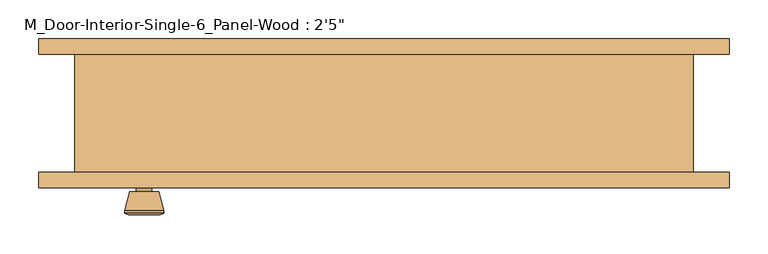
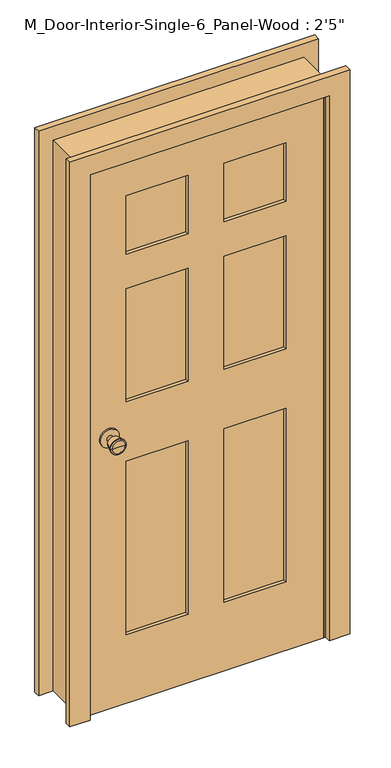
"""IFC4 building model written with IfcOpenShell, lengths in millimetres: door geometry."""

from ifc_helpers import new_model, si_unit, point, frame, frame_2d, origin, place, context, project, spatial, polyline, circle_curve, trimmed, segment, composite_curve, outline, extrude, faceted_brep, source, transform, mapped, element, save
from ifc_brep_helpers import plane_surface, cylinder_surface, revolved_surface, advanced_brep


def door_741bd24b(model_context):
    return source(origin(), model_context, "Body", "SolidModel", [
        advanced_brep(
        [(-310.0, -32.025, 914.4), (-320.0, -32.025, 914.4), (-300.0, -32.025, 914.4), (-289.5241324, 16.975, 914.4), (-330.4758676, 16.975, 914.4), (-310.0, 16.975, 914.4), (-285.0, 15.1471319, 914.4), (-335.0, 15.1471319, 914.4), (-285.0, 11.6834537, 914.4), (-335.0, 11.6834537, 914.4), (-291.363764, -13.025, 914.4), (-328.636236, -13.025, 914.4), (-300.0, -13.025, 914.4), (-320.0, -13.025, 914.4)],
        [
            (0, 1),
            (1, 2, circle_curve(frame((-310.0, -32.025, 914.4), z_axis=(0.0, -1.0, 0.0), x_axis=(-1.0, 0.0, 0.0)), 10.0)),
            (2, 0),
            (2, 1, circle_curve(frame((-310.0, -32.025, 914.4), z_axis=(0.0, -1.0, 0.0), x_axis=(-1.0, 0.0, 0.0)), 10.0)),
            (3, 4, circle_curve(frame((-310.0, 16.975, 914.4), z_axis=(0.0, 1.0, 0.0), x_axis=(-1.0, 0.0, 0.0)), 20.4758676)),
            (4, 5),
            (5, 3),
            (4, 3, circle_curve(frame((-310.0, 16.975, 914.4), z_axis=(0.0, 1.0, 0.0), x_axis=(-1.0, 0.0, 0.0)), 20.4758676)),
            (6, 7, circle_curve(frame((-310.0, 15.1471319, 914.4), z_axis=(0.0, 1.0, 0.0), x_axis=(-1.0, 0.0, 0.0)), 25.0)),
            (7, 4),
            (3, 6),
            (7, 6, circle_curve(frame((-310.0, 15.1471319, 914.4), z_axis=(0.0, 1.0, 0.0), x_axis=(-1.0, 0.0, 0.0)), 25.0)),
            (8, 9, circle_curve(frame((-310.0, 11.6834537, 914.4), z_axis=(0.0, 1.0, 0.0), x_axis=(-1.0, 0.0, 0.0)), 25.0)),
            (9, 7),
            (6, 8),
            (9, 8, circle_curve(frame((-310.0, 11.6834537, 914.4), z_axis=(0.0, 1.0, 0.0), x_axis=(-1.0, 0.0, 0.0)), 25.0)),
            (10, 11, circle_curve(frame((-310.0, -13.025, 914.4), z_axis=(0.0, 1.0, 0.0), x_axis=(-1.0, 0.0, 0.0)), 18.636236)),
            (11, 9),
            (8, 10),
            (11, 10, circle_curve(frame((-310.0, -13.025, 914.4), z_axis=(0.0, 1.0, 0.0), x_axis=(-1.0, 0.0, 0.0)), 18.636236)),
            (12, 13, circle_curve(frame((-310.0, -13.025, 914.4), z_axis=(0.0, 1.0, 0.0), x_axis=(-1.0, 0.0, 0.0)), 10.0)),
            (13, 11),
            (10, 12),
            (13, 12, circle_curve(frame((-310.0, -13.025, 914.4), z_axis=(0.0, 1.0, 0.0), x_axis=(-1.0, 0.0, 0.0)), 10.0)),
            (1, 13),
            (12, 2),
        ],
        [
            plane_surface(frame((-310.0, -32.025, 914.4), z_axis=(0.0, -1.0, 0.0), x_axis=(-1.0, 0.0, 0.0))),
            plane_surface(frame((-310.0, 16.975, 914.4), z_axis=(0.0, 1.0, 0.0), x_axis=(-1.0, 0.0, 0.0))),
            revolved_surface(polyline([(-330.4758676, 16.975, 914.4), (-335.0, 15.1471319, 914.4)]), (-310.0, -32.025, 914.4), (0.0, -1.0, 0.0)),
            cylinder_surface(frame((-310.0, -32.025, 914.4), z_axis=(0.0, -1.0, 0.0), x_axis=(-1.0, 0.0, 0.0)), 25.0),
            revolved_surface(polyline([(-335.0, 11.6834537, 914.4), (-328.636236, -13.025, 914.4)]), (-310.0, -32.025, 914.4), (0.0, -1.0, 0.0)),
            plane_surface(frame((-310.0, -13.025, 914.4), z_axis=(0.0, -1.0, 0.0), x_axis=(-1.0, 0.0, 0.0))),
            cylinder_surface(frame((-310.0, -32.025, 914.4), z_axis=(0.0, -1.0, 0.0), x_axis=(-1.0, 0.0, 0.0)), 10.0),
        ],
        [
            (0, [[1, 2, 3]]),
            (0, [[-3, 4, -1]]),
            (1, [[5, 6, 7]]),
            (1, [[8, -7, -6]]),
            (2, [[9, 10, -5, 11]]),
            (2, [[12, -11, -8, -10]]),
            (3, [[13, 14, -9, 15]]),
            (3, [[16, -15, -12, -14]]),
            (4, [[17, 18, -13, 19]]),
            (4, [[20, -19, -16, -18]]),
            (5, [[21, 22, -17, 23]]),
            (5, [[24, -23, -20, -22]]),
            (6, [[-2, 25, -21, 26]]),
            (6, [[-4, -26, -24, -25]]),
        ],
    ),
        extrude(outline(composite_curve([segment(trimmed(circle_curve(frame_2d((914.4, -310.0)), 30.0), [point((914.4, -340.0))], [point((914.4, -280.0))], False, "CARTESIAN"), True, "CONTINUOUS"), segment(trimmed(circle_curve(frame_2d((914.4, -310.0)), 30.0), [point((914.4, -280.0))], [point((914.4, -340.0))], False, "CARTESIAN"), True, "CONTINUOUS")], self_intersect=False)), frame((0.0, -38.025, 0.0), z_axis=(0.0, 1.0, 0.0), x_axis=(0.0, 0.0, 1.0)), (0.0, 0.0, 1.0), 6.0),
        advanced_brep(
        [(-310.0, -79.025, 914.4), (-300.0, -79.025, 914.4), (-320.0, -79.025, 914.4), (-289.5241324, -128.025, 914.4), (-310.0, -128.025, 914.4), (-330.4758676, -128.025, 914.4), (-285.0, -126.1971319, 914.4), (-335.0, -126.1971319, 914.4), (-285.0, -122.7334537, 914.4), (-335.0, -122.7334537, 914.4), (-291.363764, -98.025, 914.4), (-328.636236, -98.025, 914.4), (-300.0, -98.025, 914.4), (-320.0, -98.025, 914.4)],
        [
            (0, 1),
            (1, 2, circle_curve(frame((-310.0, -79.025, 914.4), z_axis=(0.0, 1.0, 0.0), x_axis=(-1.0, 0.0, 0.0)), 10.0)),
            (2, 0),
            (2, 1, circle_curve(frame((-310.0, -79.025, 914.4), z_axis=(0.0, 1.0, 0.0), x_axis=(-1.0, 0.0, 0.0)), 10.0)),
            (3, 4),
            (4, 5),
            (5, 3, circle_curve(frame((-310.0, -128.025, 914.4), z_axis=(0.0, -1.0, 0.0), x_axis=(-1.0, 0.0, 0.0)), 20.4758676)),
            (3, 5, circle_curve(frame((-310.0, -128.025, 914.4), z_axis=(0.0, -1.0, 0.0), x_axis=(-1.0, 0.0, 0.0)), 20.4758676)),
            (6, 3),
            (5, 7),
            (7, 6, circle_curve(frame((-310.0, -126.1971319, 914.4), z_axis=(0.0, -1.0, 0.0), x_axis=(-1.0, 0.0, 0.0)), 25.0)),
            (6, 7, circle_curve(frame((-310.0, -126.1971319, 914.4), z_axis=(0.0, -1.0, 0.0), x_axis=(-1.0, 0.0, 0.0)), 25.0)),
            (8, 6),
            (7, 9),
            (9, 8, circle_curve(frame((-310.0, -122.7334537, 914.4), z_axis=(0.0, -1.0, 0.0), x_axis=(-1.0, 0.0, 0.0)), 25.0)),
            (8, 9, circle_curve(frame((-310.0, -122.7334537, 914.4), z_axis=(0.0, -1.0, 0.0), x_axis=(-1.0, 0.0, 0.0)), 25.0)),
            (10, 8),
            (9, 11),
            (11, 10, circle_curve(frame((-310.0, -98.025, 914.4), z_axis=(0.0, -1.0, 0.0), x_axis=(-1.0, 0.0, 0.0)), 18.636236)),
            (10, 11, circle_curve(frame((-310.0, -98.025, 914.4), z_axis=(0.0, -1.0, 0.0), x_axis=(-1.0, 0.0, 0.0)), 18.636236)),
            (12, 10),
            (11, 13),
            (13, 12, circle_curve(frame((-310.0, -98.025, 914.4), z_axis=(0.0, -1.0, 0.0), x_axis=(-1.0, 0.0, 0.0)), 10.0)),
            (12, 13, circle_curve(frame((-310.0, -98.025, 914.4), z_axis=(0.0, -1.0, 0.0), x_axis=(-1.0, 0.0, 0.0)), 10.0)),
            (1, 12),
            (13, 2),
        ],
        [
            plane_surface(frame((-310.0, -79.025, 914.4), z_axis=(0.0, 1.0, 0.0), x_axis=(-1.0, 0.0, 0.0))),
            plane_surface(frame((-310.0, -128.025, 914.4), z_axis=(0.0, -1.0, 0.0), x_axis=(-1.0, 0.0, 0.0))),
            revolved_surface(polyline([(-330.4758676, -128.025, 914.4), (-335.0, -126.1971319, 914.4)]), (-310.0, -79.025, 914.4), (0.0, 1.0, 0.0)),
            cylinder_surface(frame((-310.0, -79.025, 914.4), z_axis=(0.0, 1.0, 0.0), x_axis=(-1.0, 0.0, 0.0)), 25.0),
            revolved_surface(polyline([(-335.0, -122.7334537, 914.4), (-328.636236, -98.025, 914.4)]), (-310.0, -79.025, 914.4), (0.0, 1.0, 0.0)),
            plane_surface(frame((-310.0, -98.025, 914.4), z_axis=(0.0, 1.0, 0.0), x_axis=(-1.0, 0.0, 0.0))),
            cylinder_surface(frame((-310.0, -79.025, 914.4), z_axis=(0.0, 1.0, 0.0), x_axis=(-1.0, 0.0, 0.0)), 10.0),
        ],
        [
            (0, [[1, 2, 3]]),
            (0, [[-3, 4, -1]]),
            (1, [[5, 6, 7]]),
            (1, [[-6, -5, 8]]),
            (2, [[9, -7, 10, 11]]),
            (2, [[-10, -8, -9, 12]]),
            (3, [[13, -11, 14, 15]]),
            (3, [[-14, -12, -13, 16]]),
            (4, [[17, -15, 18, 19]]),
            (4, [[-18, -16, -17, 20]]),
            (5, [[21, -19, 22, 23]]),
            (5, [[-22, -20, -21, 24]]),
            (6, [[25, -23, 26, -2]]),
            (6, [[-26, -24, -25, -4]]),
        ],
    ),
        extrude(outline(composite_curve([segment(trimmed(circle_curve(frame_2d((914.4, -310.0)), 30.0), [point((914.4, -340.0))], [point((914.4, -280.0))], False, "CARTESIAN"), True, "CONTINUOUS"), segment(trimmed(circle_curve(frame_2d((914.4, -310.0)), 30.0), [point((914.4, -280.0))], [point((914.4, -340.0))], False, "CARTESIAN"), True, "CONTINUOUS")], self_intersect=False)), frame((0.0, -79.025, 0.0), z_axis=(0.0, 1.0, 0.0), x_axis=(0.0, 0.0, 1.0)), (0.0, 0.0, 1.0), 6.0),
        faceted_brep([(400.0, -73.025, 0.0), (375.0, -73.025, 0.0), (375.0, -38.025, 0.0), (362.3, -38.025, 0.0), (362.3, -3.1, 0.0), (375.0, -3.1, 0.0), (375.0, 79.375, 0.0), (400.0, 79.375, 0.0), (400.0, 79.375, 1853.8), (400.0, -73.025, 1853.8), (375.0, 79.375, 1828.8), (-375.0, 79.375, 1828.8), (-375.0, 79.375, 0.0), (-400.0, 79.375, 0.0), (-400.0, 79.375, 1853.8), (375.0, -3.1, 1828.8), (362.3, -3.1, 1816.1), (-362.3, -3.1, 1816.1), (-362.3, -3.1, 0.0), (-375.0, -3.1, 0.0), (-375.0, -3.1, 1828.8), (362.3, -38.025, 1816.1), (375.0, -38.025, 1828.8), (-375.0, -38.025, 1828.8), (-375.0, -38.025, 0.0), (-362.3, -38.025, 0.0), (-362.3, -38.025, 1816.1), (375.0, -73.025, 1828.8), (-400.0, -73.025, 1853.8), (-400.0, -73.025, 0.0), (-375.0, -73.025, 0.0), (-375.0, -73.025, 1828.8)], [[[0, 1, 2, 3, 4, 5, 6, 7]], [[7, 8, 9, 0]], [[6, 10, 11, 12, 13, 14, 8, 7]], [[5, 15, 10, 6]], [[4, 16, 17, 18, 19, 20, 15, 5]], [[3, 21, 16, 4]], [[2, 22, 23, 24, 25, 26, 21, 3]], [[1, 27, 22, 2]], [[0, 9, 28, 29, 30, 31, 27, 1]], [[8, 14, 28, 9]], [[15, 20, 11, 10]], [[21, 26, 17, 16]], [[27, 31, 23, 22]], [[29, 13, 12, 19, 18, 25, 24, 30]], [[14, 13, 29, 28]], [[20, 19, 12, 11]], [[26, 25, 18, 17]], [[31, 30, 24, 23]]]),
        extrude(outline(polyline([(1828.8, -375.0), (0.0, -375.0), (0.0, 375.0), (1828.8, 375.0), (1828.8, -375.0)]), holes=[polyline([(1708.8, 57.5), (1708.8, 255.0), (1511.3, 255.0), (1511.3, 57.5), (1708.8, 57.5)]), polyline([(1396.3, 255.0), (1014.4, 255.0), (1014.4, 57.5), (1396.3, 57.5), (1396.3, 255.0)]), polyline([(1014.4, -57.5), (1014.4, -255.0), (1396.3, -255.0), (1396.3, -57.5), (1014.4, -57.5)]), polyline([(1511.3, -255.0), (1708.8, -255.0), (1708.8, -57.5), (1511.3, -57.5), (1511.3, -255.0)]), polyline([(814.4, 57.5), (814.4, 255.0), (230.0, 255.0), (230.0, 57.5), (814.4, 57.5)]), polyline([(230.0, -57.5), (230.0, -255.0), (814.4, -255.0), (814.4, -57.5), (230.0, -57.5)])]), frame((0.0, -73.025, 0.0), z_axis=(0.0, 1.0, 0.0), x_axis=(0.0, 0.0, 1.0)), (0.0, 0.0, 1.0), 35.0),
        extrude(outline(polyline([(255.0, -49.6916667), (255.0, -61.3583333), (57.5, -61.3583333), (57.5, -49.6916667), (255.0, -49.6916667)])), frame((0.0, 0.0, 1511.3), z_axis=(0.0, 0.0, 1.0), x_axis=(1.0, 0.0, 0.0)), (0.0, 0.0, 1.0), 197.5),
        extrude(outline(polyline([(255.0, -49.6916667), (255.0, -61.3583333), (57.5, -61.3583333), (57.5, -49.6916667), (255.0, -49.6916667)])), frame((0.0, 0.0, 1014.4), z_axis=(0.0, 0.0, 1.0), x_axis=(1.0, 0.0, 0.0)), (0.0, 0.0, 1.0), 381.9),
        extrude(outline(polyline([(-57.5, -49.6916667), (-57.5, -61.3583333), (-255.0, -61.3583333), (-255.0, -49.6916667), (-57.5, -49.6916667)])), frame((0.0, 0.0, 1014.4), z_axis=(0.0, 0.0, 1.0), x_axis=(1.0, 0.0, 0.0)), (0.0, 0.0, 1.0), 381.9),
        extrude(outline(polyline([(-57.5, -49.6916667), (-57.5, -61.3583333), (-255.0, -61.3583333), (-255.0, -49.6916667), (-57.5, -49.6916667)])), frame((0.0, 0.0, 1511.3), z_axis=(0.0, 0.0, 1.0), x_axis=(1.0, 0.0, 0.0)), (0.0, 0.0, 1.0), 197.5),
        extrude(outline(polyline([(255.0, -49.6916667), (255.0, -61.3583333), (57.5, -61.3583333), (57.5, -49.6916667), (255.0, -49.6916667)])), frame((0.0, 0.0, 230.0), z_axis=(0.0, 0.0, 1.0), x_axis=(1.0, 0.0, 0.0)), (0.0, 0.0, 1.0), 584.4),
        extrude(outline(polyline([(-57.5, -49.6916667), (-57.5, -61.3583333), (-255.0, -61.3583333), (-255.0, -49.6916667), (-57.5, -49.6916667)])), frame((0.0, 0.0, 230.0), z_axis=(0.0, 0.0, 1.0), x_axis=(1.0, 0.0, 0.0)), (0.0, 0.0, 1.0), 584.4),
        extrude(outline(polyline([(0.0, 446.35), (1900.15, 446.35), (1900.15, -446.35), (0.0, -446.35), (0.0, -381.35), (1835.15, -381.35), (1835.15, 381.35), (0.0, 381.35), (0.0, 446.35)])), frame((0.0, -93.025, 0.0), z_axis=(0.0, 1.0, 0.0), x_axis=(0.0, 0.0, 1.0)), (0.0, 0.0, 1.0), 20.0),
        extrude(outline(polyline([(0.0, 446.35), (1900.15, 446.35), (1900.15, -446.35), (0.0, -446.35), (0.0, -381.35), (1835.15, -381.35), (1835.15, 381.35), (0.0, 381.35), (0.0, 446.35)])), frame((0.0, 79.375, 0.0), z_axis=(0.0, 1.0, 0.0), x_axis=(0.0, 0.0, 1.0)), (0.0, 0.0, 1.0), 20.0),
    ])


if __name__ == "__main__":
    model = new_model("IFC4")
    model_context = context("Model", 3, world=origin())
    ifc_project = project(units=[si_unit("LENGTHUNIT", "METRE", prefix="MILLI")], contexts=[model_context])
    site = spatial("IfcSite", under=ifc_project)
    building = spatial("IfcBuilding", under=site)
    placement = place(None, origin())
    door_shape = door_741bd24b(model_context)
    element("IfcDoor", 1, ObjectType="M_Door-Interior-Single-6_Panel-Wood : 2'5\"", at=placement, inside=building, context=model_context, shape_type="MappedRepresentation", body=[
        mapped(door_shape, transform((0.0, 0.0, 0.0), x_axis=(1.0, 0.0, 0.0), y_axis=(0.0, 1.0, 0.0), z_axis=(0.0, 0.0, 1.0))),
    ])
    save(model, "model.ifc")

# Revit data of these elements
# Type "M_Door-Interior-Single-6_Panel-Wood : 2'5\""
#   Type Mark = "11"
#   Assembly Code = "C1020300"
#   Analytic Construction = "Wooden"
#   Top Rail = 0' - 4.72441"
#   Top Panel = 0' - 7.77559"
#   Thickness = 0' - 1.37795"
#   Thermal Resistance (R) = 2.5876 (h·ft²·°F)/BTU
#   Swing Angle [instance default] = 90.00°
#   Stiles = 0' - 4.72441"
#   Rough Width = 2' - 7.49606"
#   Rough Height = 6' - 0.98425"
#   Mullion = 0' - 4.52756"
#   Lock Rail = 0' - 7.87402"
#   Intermediate Rail = 0' - 4.52756"
#   Height = 6' - 0"
#   Width = 2' - 5.52756"
#   Heat Transfer Coefficient (U) = 0.3865 BTU/(h·ft²·°F)
#   Bottom Rail = 0' - 9.05512"
#   Trim Material = Cherry
#   Panel Material = Cherry
#   Frame Material = Cherry
#   Door Handle Material = Aluminum
#   Visual Light Transmittance = 0
#   Solar Heat Gain Coefficient = 0
#   Wall Closure = (empty or 0)
#   Function = (empty or 0)
# Element 1 (IfcDoor, "M_Door-Interior-Single-6_Panel-Wood : 2'5\"")
#   Materials on its faces: "Cherry", "Aluminum"
# Materials
#   "Cherry": class "Wood", colour RGB 226 177 128, transparency 0, Description = "Prunus Serotina", Cost = 0
#   "Aluminum": class "Metal", colour RGB 247 247 247, transparency 0, Description = "Aluminum 6061", Cost = 0
